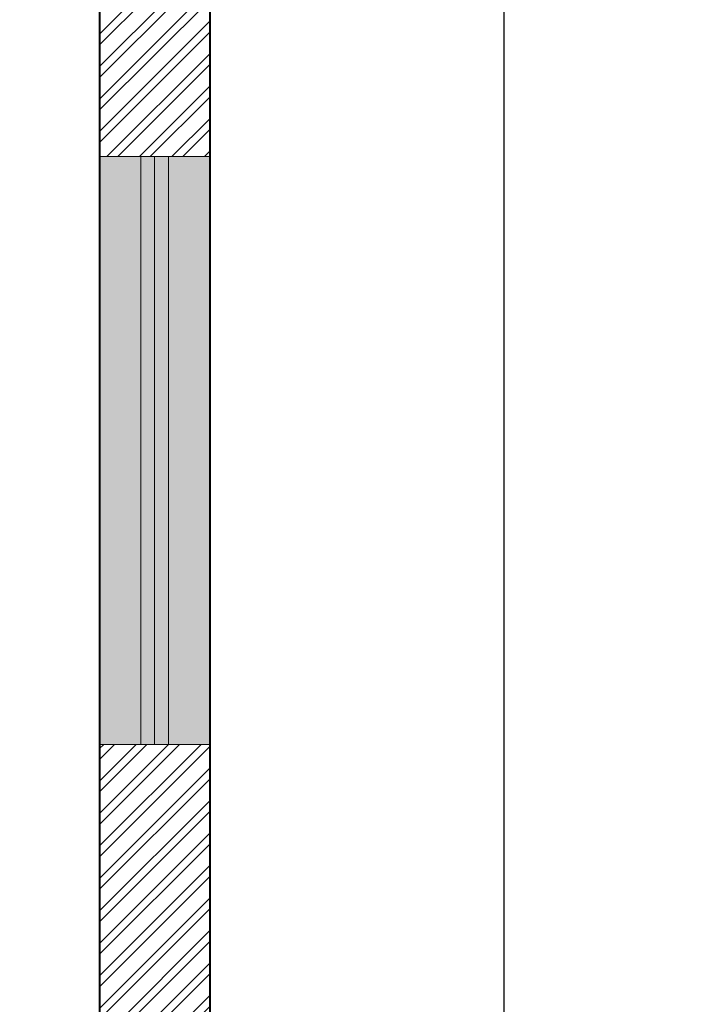
# Model space of a CAD drawing. Units: inches. Extents: x 528 to 2520, y -151 to 1354.
# Tile 13 of 41: x 870 to 924, y 1150 to 1231. Entities that reach past the tile are written whole.
import ezdxf

# ---------------------------------------------------------------- set-up
doc = ezdxf.new("R2010")
doc.units = ezdxf.units.IN
doc.header["$MEASUREMENT"] = 0
for name, color, linetype, lineweight in [('A-ANNO-DIMS', 2, 'Continuous', 18), ('A-WALL-PATT', 6, 'Continuous', 13), ('walls', 7, 'Continuous', 40), ('WINDOWS', 2, 'Continuous', 20)]:
    doc.layers.add(name, color=color, linetype=linetype, lineweight=lineweight)
doc.layers.add('A-GLAZ-PATT', color=152, linetype='Continuous', lineweight=13, true_color=0x2776bb)
doc.styles.get("Standard").update_dxf_attribs({"font": 'arial.ttf'})
doc.dimstyles.get("Standard").update_dxf_attribs({"dimtxt": 6, "dimasz": 2, "dimexe": 0.18, "dimexo": 0.0625, "dimgap": 0.09, "dimtad": 0, "dimtih": 1, "dimtoh": 1, "dimdec": 1, "dimzin": 0, "dimdsep": 46, "dimlunit": 3, "dimtxsty": 'Standard', "dimblk": 'ARCHTICK', "dimcen": 0.09, "dimadec": 0, "dimazin": 0, "dimtfac": 1, "dimtdec": 1, "dimtofl": 0, "dimtmove": 0, "dimatfit": 3, "dimfxl": 1, "dimtolj": 1, "dimtzin": 0, "dimarcsym": 0})

# ---------------------------------------------------------------- blocks, each defined once
blk = doc.blocks.new('_ArchTick')
at = {"color": 0, "linetype": 'ByBlock', "const_width": 0.15}
blk.add_lwpolyline([(-0.5, -0.5), (0.5, 0.5)], dxfattribs=at)
blk = doc.blocks.new('*D24')
at = {"layer": 'A-ANNO-DIMS', "color": 0, "lineweight": -2, "transparency": 16777216}
for p, q in [((885.759, 1317.103), (909.9, 1317.103)), ((909.72, 1317.103), (909.72, 1069.756)), ((909.72, 816.103), (909.72, 1063.449)), ((885.759, 816.103), (909.9, 816.103))]:
    blk.add_line(p, q, dxfattribs=at)
at = {"layer": 'Defpoints', "color": 0, "transparency": 16777216}
for p in [(885.697, 1317.103), (885.697, 816.103), (909.72, 816.103)]:
    blk.add_point(p, dxfattribs=at)
at = {"layer": 'A-ANNO-DIMS', "color": 0, "lineweight": -2, "transparency": 16777216, "xscale": 2, "yscale": 2, "zscale": 2}
for p, rotation in [((909.72, 1317.103), 90), ((909.72, 816.103), 270)]:
    blk.add_blockref('_ArchTick', p, dxfattribs=dict(at, rotation=rotation))
at = {"layer": 'A-ANNO-DIMS', "color": 0, "transparency": 16777216, "insert": (909.72, 1066.603), "char_height": 6, "attachment_point": 5}
blk.add_mtext('\\A1;41\'-9.0"', dxfattribs=at)
blk = doc.blocks.new('WINDOW-48x9-PLAN')
for p, q in [((0, 5.632), (48, 5.632)), ((0, 4.5), (48, 4.5)), ((0, 3.368), (48, 3.368))]:
    blk.add_line(p, q)
blk.add_lwpolyline([(0, 9), (48, 9), (48, 0), (0, 0)], close=True)

msp = doc.modelspace()

# ---------------------------------------------------------------- hatches: boundary and pattern name
at = {"layer": 'A-GLAZ-PATT'}
h = msp.add_hatch(color=256, dxfattribs=at)
h.dxf.hatch_style = 1
h.paths.add_polyline_path([(876.697, 1219.369), (876.697, 1171.369), (880.065, 1171.369), (880.065, 1219.369)])
h.paths.add_polyline_path([(880.065, 1219.369), (880.065, 1171.369), (881.197, 1171.369), (881.197, 1219.369)])
h.paths.add_polyline_path([(881.197, 1219.369), (881.197, 1171.369), (882.328, 1171.369), (882.328, 1219.369)])
h.paths.add_polyline_path([(882.328, 1219.369), (882.328, 1171.369), (885.697, 1171.369), (885.697, 1219.369)])
at = {"layer": 'A-WALL-PATT'}
h = msp.add_hatch(dxfattribs=at)
h.set_pattern_fill('ANSI32', color=256, scale=5)
h.paths.add_polyline_path([(595.697, 1163.855), (586.697, 1163.855), (586.697, 969.103), (598.244, 969.103), (603.244, 969.103), (603.244, 974.103), (595.697, 974.103), (595.697, 1082.103), (691.697, 1082.103), (691.697, 1087.103), (691.697, 1106.103), (697.697, 1106.103), (697.697, 1111.103), (686.697, 1111.103), (686.697, 1087.103), (595.697, 1087.103)])
h.paths.add_polyline_path([(688.702, 974.103), (651.244, 974.103), (651.244, 969.103), (688.702, 969.103)])
h.paths.add_polyline_path([(885.697, 1171.369), (876.697, 1171.369), (876.697, 1111.103), (786.697, 1111.103), (786.697, 1106.103), (876.697, 1106.103), (876.697, 974.103), (786.697, 974.103), (786.697, 969.103), (876.697, 969.103), (876.697, 825.103), (834.697, 825.103), (834.697, 816.103), (885.697, 816.103)])
h.paths.add_polyline_path([(885.697, 1317.103), (876.652, 1317.103), (876.652, 1308.103), (876.697, 1308.103), (876.697, 1248.103), (822.697, 1248.103), (822.697, 1243.103), (876.697, 1243.103), (876.697, 1219.369), (885.697, 1219.369)])
h.paths.add_polyline_path([(852.652, 1317.103), (787.697, 1317.103), (787.697, 1248.103), (784.263, 1248.103), (784.263, 1243.103), (792.697, 1243.103), (792.697, 1249.103), (792.697, 1308.103), (852.652, 1308.103)])
h.paths.add_polyline_path([(684.697, 1317.103), (619.697, 1317.103), (619.697, 1308.103), (679.697, 1308.103), (679.697, 1248.103), (679.697, 1243.103), (684.697, 1243.103), (684.697, 1248.248)])
h.paths.add_polyline_path([(595.697, 1308.103), (595.697, 1317.103), (586.697, 1317.103), (586.697, 1211.855), (595.697, 1211.855), (595.697, 1243.103), (649.697, 1243.103), (649.697, 1248.103), (595.697, 1248.103)])
h.paths.add_polyline_path([(744.697, 969.103), (744.697, 974.103), (724.702, 974.103), (724.702, 969.103), (739.697, 969.103), (739.697, 874.287), (744.697, 874.287)])
h.paths.add_polyline_path([(739.697, 969.103), (727.697, 969.103), (727.697, 965.117), (730.735, 965.117), (730.735, 961.676), (734.434, 961.676), (734.434, 957.24), (739.697, 957.24)], flags=17)
h.paths.add_polyline_path([(786.697, 825.103), (744.697, 825.103), (744.697, 832.287), (739.697, 832.287), (739.697, 816.103), (786.697, 816.103)])

# ---------------------------------------------------------------- linework, layer by layer
at = {"layer": 'walls'}
for p, q in [((885.697, 1317.103), (885.697, 816.103)), ((876.697, 1243.103), (876.697, 1111.103))]:
    msp.add_line(p, q, dxfattribs=at)

# ---------------------------------------------------------------- block references
at = {"layer": 'WINDOWS', "rotation": 89.99999999999982}
msp.add_blockref('WINDOW-48x9-PLAN', (885.696, 1171.369), dxfattribs=at)

# ---------------------------------------------------------------- dimensions: what is measured, and where the dimension line sits
at = {"layer": 'A-ANNO-DIMS'}
dim = msp.add_linear_dim(base=(909.72, 816.103), p1=(885.697, 1317.103), p2=(885.697, 816.103), angle=90, dimstyle='Standard', override={"dimclrd": 0, "dimclre": 0, "dimclrt": 0}, dxfattribs=at)
dim.commit()
dim.dimension.update_dxf_attribs({"geometry": '*D24', "text_midpoint": (909.72, 1066.603)})

doc.saveas('drawing.dxf')
